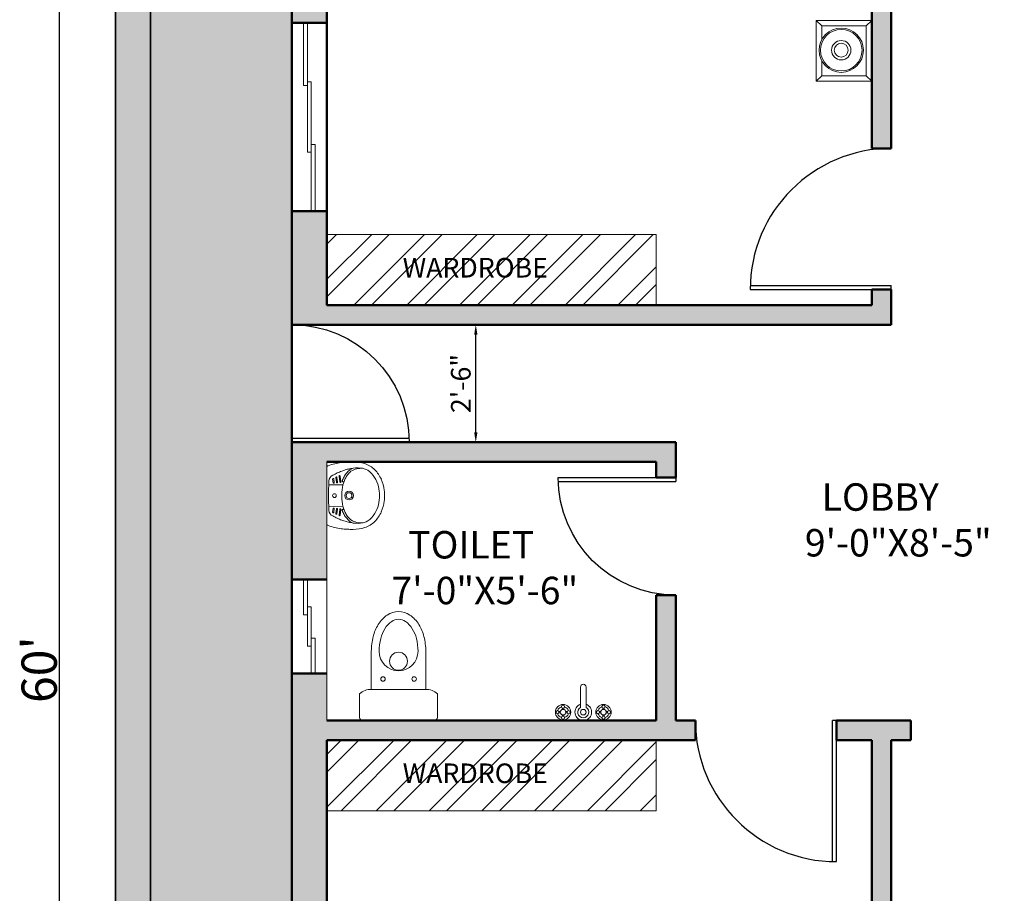
# Model space of a CAD drawing. Units: inches. Extents: x 1734 to 4011, y 1071 to 1891.
# Tile 3 of 27: x 1734 to 1985, y 1427 to 1650. Entities that reach past the tile are written whole.
import ezdxf

# ---------------------------------------------------------------- set-up
doc = ezdxf.new("R2010")
doc.units = ezdxf.units.IN
for name, color, linetype, lineweight in [('0.15', 34, 'Continuous', 15), ('A-ANNO-DIMS', 2, 'Continuous', 18), ('A-AREA-IDEN', 3, 'Continuous', 18), ('A-DOOR', 3, 'Continuous', 25), ('A-FLOR-FIXT', 9, 'Continuous', 18), ('A-FLOR-PATT', 252, 'Continuous', 13), ('A-FURN', 8, 'Continuous', 18), ('A-FURN-PATT', 252, 'Continuous', 13), ('A-GLAZ', 4, 'Continuous', 18), ('A-WALL', 7, 'Continuous', 50), ('A-WALL-PATT', 8, 'Continuous', 13), ('C-PROP', 1, 'Continuous', 35)]:
    doc.layers.add(name, color=color, linetype=linetype, lineweight=lineweight)
doc.styles.get("Standard").update_dxf_attribs({"font": 'arial.ttf'})
doc.dimstyles.new('ISO-25', dxfattribs={"dimtxt": 5, "dimasz": 2.5, "dimexe": 1.25, "dimexo": 0.625, "dimtad": 1, "dimdec": 1, "dimlunit": 3, "dimtxsty": 'Standard', "dimcen": 2.5, "dimclrt": 1, "dimadec": 0, "dimazin": 0, "dimtfac": 1, "dimtdec": 1, "dimtmove": 0, "dimatfit": 3, "dimfxl": 1, "dimarcsym": 0})

# ---------------------------------------------------------------- blocks, each defined once
blk = doc.blocks.new('*D1')
at = {"layer": 'A-ANNO-DIMS', "color": 0, "lineweight": -2, "transparency": 16777216}
for p, q in [((1850.54, 1572.06), (1849.37, 1572.06)), ((1850.62, 1544.56), (1850.62, 1569.56)), ((1850.54, 1542.06), (1849.37, 1542.06))]:
    blk.add_line(p, q, dxfattribs=at)
at = {"layer": 'A-ANNO-DIMS', "color": 0, "transparency": 16777216}
for points in [[(1850.21, 1569.56), (1851.04, 1569.56), (1850.62, 1572.06)], [(1850.21, 1544.56), (1851.04, 1544.56), (1850.62, 1542.06)]]:
    blk.add_solid(points, dxfattribs=at)
at = {"layer": 'Defpoints', "color": 0, "transparency": 16777216}
for p in [(1850.62, 1572.06), (1851.16, 1572.06), (1851.16, 1542.06)]:
    blk.add_point(p, dxfattribs=at)
at = {"layer": 'A-ANNO-DIMS', "color": 0, "transparency": 16777216, "insert": (1847.45, 1557.06), "char_height": 5, "attachment_point": 5, "rotation": 90}
blk.add_mtext('2\'-6"', dxfattribs=at)
blk = doc.blocks.new('*D15')
at = {"layer": 'A-ANNO-DIMS', "color": 0, "lineweight": -2, "transparency": 16777216}
for p, q in [((1758.02, 1844.06), (1743.18, 1844.06)), ((1744.43, 1126.56), (1744.43, 1841.56)), ((1758.02, 1124.06), (1743.18, 1124.06))]:
    blk.add_line(p, q, dxfattribs=at)
at = {"layer": 'A-ANNO-DIMS', "color": 0, "transparency": 16777216}
for points in [[(1744.01, 1841.56), (1744.84, 1841.56), (1744.43, 1844.06)], [(1744.01, 1126.56), (1744.84, 1126.56), (1744.43, 1124.06)]]:
    blk.add_solid(points, dxfattribs=at)
at = {"layer": 'Defpoints', "color": 0, "transparency": 16777216}
for p in [(1744.43, 1844.06), (1758.65, 1844.06), (1758.65, 1124.06)]:
    blk.add_point(p, dxfattribs=at)
at = {"layer": 'A-ANNO-DIMS', "color": 0, "transparency": 16777216, "insert": (1739.21, 1484.06), "char_height": 5, "attachment_point": 5, "rotation": 90}
blk.add_mtext("{\\H1.8x;60'}", dxfattribs=at)
blk = doc.blocks.new("D1 3'")
for p, q in [((0, 36), (0, 0)), ((1, 36), (1, 0)), ((0, 0), (1, 0))]:
    blk.add_line(p, q)
blk.add_arc((0, 0), 36, 0, 90)
blk = doc.blocks.new("D2 2'6")
for p, q in [((0, 30), (0, 0)), ((1, 30), (1, 0)), ((0, 0), (1, 0))]:
    blk.add_line(p, q)
blk.add_arc((0, 0), 30, 0, 90)
blk = doc.blocks.new('VELADOR')
at = {"layer": '0.15'}
for p, q in [((-0.2475, 0), (-0.2025, -0.045)), ((0.2475, 0), (0.2025, -0.045)), ((-0.2025, -0.405), (-0.2475, -0.45)), ((0.2475, -0.45), (0.2025, -0.405))]:
    blk.add_line(p, q, dxfattribs=at)
blk.add_lwpolyline([(-0.2475, 0), (-0.2475, -0.45), (0.2475, -0.45), (0.2475, 0)], close=True, dxfattribs=at)
blk.add_lwpolyline([(0.0921, -0.405), (0.2025, -0.405), (0.2025, -0.045), (-0.2025, -0.045), (-0.2025, -0.405), (-0.0818, -0.405)], dxfattribs=at)
for radius in [0.18, 0.1688, 0.0788, 0.0563]:
    blk.add_circle((0.0052, -0.2474), radius, dxfattribs=at)
blk = doc.blocks.new('lavamanos 2')
at = {"layer": '0.15'}
for p, q in [((0, 0.2335), (0, -0.2335)), ((-0.1304, 0.11), (-0.1315, 0.11)), ((-0.0142, 0.087), (-0.13, 0.086)), ((-0.1127, 0.112), (-0.1067, 0.1581)), ((-0.1037, 0.1109), (-0.0978, 0.157)), ((-0.0857, 0.1085), (-0.0807, 0.1466)), ((-0.0767, 0.1074), (-0.0718, 0.1455)), ((-0.0587, 0.105), (-0.0548, 0.1351)), ((-0.0497, 0.1039), (-0.0458, 0.134)), ((-0.1304, -0.11), (-0.1315, -0.11)), ((-0.0142, -0.087), (-0.13, -0.086)), ((-0.1127, -0.112), (-0.1067, -0.1581)), ((-0.1037, -0.1109), (-0.0978, -0.157)), ((-0.0857, -0.1085), (-0.0807, -0.1466)), ((-0.0767, -0.1074), (-0.0718, -0.1455)), ((-0.0587, -0.105), (-0.0548, -0.1351)), ((-0.0497, -0.1039), (-0.0458, -0.134))]:
    blk.add_line(p, q, dxfattribs=at)
for centre, radius in [((-0.178, 0), 0.035), ((-0.178, 0), 0.0235), ((-0.06, 0), 0.015)]:
    blk.add_circle(centre, radius, dxfattribs=at)
for centre, radius, start, end in [((-0.2419, 0.0663), 0.2023, 108.1945, 135.36859), ((-0.2035, -0.0862), 0.3593, 91.20299, 106.42552), ((-0.2208, -0.6855), 0.9585, 86.55138, 89.41308), ((-0.2121, -0.5476), 0.8204, 83.12241, 86.5796), ((5.8279, 30.215), 30.5319, 258.77821, 258.87599), ((-0.1265, -0.0657), 0.3287, 69.06009, 78.82181), ((-0.0202, 0.212), 0.0314, 54.79491, 69.06009), ((-0.1663, 0.0005), 0.3024, 136.57187, 154.32772), ((-0.2422, 0.0655), 0.1638, 121.99295, 150.58892), ((-0.2657, 0.1037), 0.119, 92.47742, 122.14108), ((-0.2765, 0.0677), 0.1528, 57.2491, 95.54005), ((-0.2442, -0.0128), 0.2368, 77.24819, 96.46321), ((-0.2765, 0.0677), 0.1678, 56.87663, 64.99714), ((-0.3662, -0.002), 0.2627, 40.35252, 49.00458), ((-0.2222, 0.0026), 0.2177, 71.98488, 82.01242), ((-0.3662, -0.002), 0.2777, 40.35252, 49.22548), ((-0.2374, 0.11), 0.0921, 27.31862, 39.11562), ((-0.3103, -0.315), 0.5472, 69.51913, 73.49118), ((-0.2374, 0.11), 0.1071, 27.57433, 39.11562), ((-0.3494, 0.0363), 0.2408, 22.19214, 30.78376), ((-0.2991, -0.2855), 0.5156, 65.23004, 69.53785), ((-0.1022, 0.1575), 0.0045, 352.61396, 172.61396), ((-0.2784, -0.2408), 0.4663, 60.24131, 65.2382), ((-0.0648, 0.1184), 0.049, 1.58272, 68.62081), ((-0.005, 0.2335), 0.005, 0, 54.79491), ((-0.0557, -0.0178), 0.4111, 158.70106, 171.31016), ((-0.1999, 0.0263), 0.2202, 147.11565, 167.44248), ((-0.3494, 0.0363), 0.2258, 22.33605, 30.8927), ((-1.2664, -0.2389), 1.1824, 16.36313, 17.77674), ((-0.1315, 0.117), 0.007, 197.40991, 270.49494), ((0.1853, 0.1648), 0.325, 192.53887, 196.70718), ((-0.1305, 0.117), 0.007, 270.49494, 17.39527), ((-1.2664, -0.2389), 1.1974, 17.39527, 17.80495), ((-0.1082, 0.1115), 0.0045, 172.61396, 352.61396), ((-0.0812, 0.108), 0.0045, 172.61396, 352.61396), ((-0.0763, 0.146), 0.0045, 352.61396, 172.61396), ((-0.0542, 0.1045), 0.0045, 172.61396, 352.61396), ((-0.0503, 0.1345), 0.0045, 352.61396, 172.61396), ((-2.1477, 0.0009), 2.1352, 359.97535, 3.19009), ((-0.2093, 0.0056), 0.2558, 171.31016, 181.26266), ((-0.2093, -0.0056), 0.2558, 178.73734, 188.68984), ((0.4664, -0.0834), 0.8953, 169.86317, 174.65802), ((0.4664, 0.0834), 0.8953, 185.34198, 190.13683), ((0.3887, 0.121), 0.517, 185.50529, 189.81306), ((-0.7181, -0.0071), 0.5987, 0.67647, 3.82165), ((-0.7181, 0.0071), 0.5987, 356.17835, 359.32353), ((-2.1477, -0.0009), 2.1352, 356.80991, 0.02465), ((-0.0557, 0.0178), 0.4111, 188.68984, 201.29894), ((-0.1999, -0.0263), 0.2202, 192.55752, 212.88435), ((0.1853, -0.1648), 0.325, 163.29282, 167.46113), ((0.3887, -0.1209), 0.517, 170.18694, 174.49471), ((-0.1663, -0.0005), 0.3024, 205.67228, 223.42813), ((-0.2422, -0.0655), 0.1638, 209.41108, 238.00705), ((-0.2374, -0.1099), 0.0921, 320.88438, 332.68138), ((-0.3494, -0.0363), 0.2258, 329.1073, 337.66395), ((-0.3494, -0.0363), 0.2408, 329.21624, 337.80786), ((-1.2664, 0.2389), 1.1824, 342.22326, 343.63687), ((-0.1315, -0.117), 0.007, 89.50506, 162.59009), ((-0.1305, -0.117), 0.007, 342.60473, 89.50506), ((-1.2664, 0.2389), 1.1974, 342.19505, 342.60473), ((-0.1082, -0.1115), 0.0045, 7.38604, 187.38604), ((-0.1022, -0.1575), 0.0045, 187.38604, 7.38604), ((-0.0812, -0.108), 0.0045, 7.38604, 187.38604), ((-0.0763, -0.146), 0.0045, 187.38604, 7.38604), ((-0.0542, -0.1045), 0.0045, 7.38604, 187.38604), ((-0.0503, -0.1345), 0.0045, 187.38604, 7.38604), ((-0.0648, -0.1184), 0.049, 291.37919, 358.41728), ((-0.2419, -0.0663), 0.2023, 224.63141, 251.8055), ((-0.2657, -0.1036), 0.119, 237.85892, 267.52258), ((-0.2765, -0.0677), 0.1528, 264.45995, 302.7509), ((-0.2442, 0.0128), 0.2368, 263.53679, 282.75181), ((-0.2765, -0.0677), 0.1678, 295.00286, 303.12337), ((-0.3662, 0.002), 0.2627, 310.99542, 319.64748), ((-0.2222, -0.0026), 0.2177, 277.98758, 288.01512), ((-0.3662, 0.002), 0.2777, 310.77452, 319.64748), ((-0.3103, 0.315), 0.5472, 286.50882, 290.48087), ((-0.2374, -0.1099), 0.1071, 320.88438, 332.42567), ((-0.2991, 0.2855), 0.5156, 290.46215, 294.76996), ((-0.2784, 0.2408), 0.4663, 294.7618, 299.75869), ((-0.0202, -0.212), 0.0314, 290.93991, 305.20509), ((-0.005, -0.2335), 0.005, 305.20509, 0), ((-0.2035, 0.0862), 0.3593, 253.57448, 268.79701), ((-0.2208, 0.6855), 0.9585, 270.58692, 273.44862), ((-0.2121, 0.5476), 0.8204, 273.4204, 276.87759), ((5.8279, -30.215), 30.5319, 101.12401, 101.22179), ((-0.1265, 0.0657), 0.3287, 281.17819, 290.93991)]:
    blk.add_arc(centre, radius, start, end, dxfattribs=at)
blk = doc.blocks.new('rreerr')
blk.add_lwpolyline([(2512.8529, 833.5601, 0.205217), (2512.9279, 833.5883), (2512.9279, 833.7401, 0.414214), (2512.9079, 833.7601), (2512.4479, 833.7601, 0.414214), (2512.4279, 833.7401), (2512.4279, 833.5883, 0.205217), (2512.5029, 833.5601)], format="xyb")
for points in [[(2512.5468, 833.1438, 0.107027), (2512.6056, 833.0819, 0.150548), (2512.6779, 833.0596, 0.150548), (2512.7502, 833.0819, 0.107027), (2512.809, 833.1438, 0.075071), (2512.8412, 833.2206, 0.0618), (2512.8529, 833.3151), (2512.8529, 833.5601), (2512.5029, 833.5601), (2512.5029, 833.3151, 0.0618), (2512.5146, 833.2206, 0.075071)], [(2512.5631, 833.2328, 0.075071), (2512.5895, 833.1698, 0.107027), (2512.6338, 833.1232, 0.150548), (2512.6779, 833.1096, 0.150548), (2512.722, 833.1232, 0.107027), (2512.7663, 833.1698, 0.075071), (2512.7927, 833.2328, 0.0618), (2512.8029, 833.3151, 1), (2512.5529, 833.3151, 0.0618)]]:
    blk.add_lwpolyline(points, format="xyb", close=True)
for centre, radius in [((2512.5779, 833.493), 0.0146), ((2512.7779, 833.493), 0.0146), ((2512.6775, 833.3793), 0.0579)]:
    blk.add_circle(centre, radius)
blk = doc.blocks.new('Faucet - Bathroom top')
for p, q in [((-4.107, 0.125), (-4.375, 0.125)), ((-3.75, 0.4788), (-3.75, 0.75)), ((-3.5, 0.482), (-3.5, 0.75)), ((-3.1461, 0.125), (-2.875, 0.125)), ((3.143, 0.125), (2.875, 0.125)), ((3.5, 0.4788), (3.5, 0.75)), ((3.75, 0.482), (3.75, 0.75)), ((4.1039, 0.125), (4.375, 0.125)), ((-4.1039, -0.125), (-4.375, -0.125)), ((-3.75, -0.4821), (-3.75, -0.75)), ((-3.5, -0.4789), (-3.5, -0.75)), ((-3.143, -0.125), (-2.875, -0.125)), ((-0.5, -0.8639), (-0.5, -4.5)), ((0.5, -4.5), (0.5, -0.8631)), ((3.1461, -0.125), (2.875, -0.125)), ((3.5, -0.4821), (3.5, -0.75)), ((3.75, -0.4789), (3.75, -0.75)), ((4.107, -0.125), (4.375, -0.125))]:
    blk.add_line(p, q)
for centre, radius in [((-3.625, 0), 1.375), ((-4.625, 0), 0.2795), ((-3.625, 0), 0.5), ((-3.625, 1), 0.2795), ((-2.625, 0), 0.2795), ((0, 0), 0.5), ((3.625, 0), 1.375), ((2.625, 0), 0.2795), ((3.625, 0), 0.5), ((3.625, 1), 0.2795), ((4.625, 0), 0.2795), ((-3.625, -1), 0.2795), ((3.625, -1), 0.2795)]:
    blk.add_circle(centre, radius)
for centre, radius, start, end in [((-3.625, 0), 1, 105.2407, 164.2093), ((-3.625, 0), 1, 16.44125, 74.07887), ((0, 0), 1.5, 289.6514, 250.3603), ((0, 0), 1, 300.3431, 239.7554), ((3.625, 0), 1, 106.12, 164.0884), ((3.625, 0), 1, 16.23422, 73.90469), ((-3.625, 0), 1, 196.2342, 253.9047), ((-3.625, 0), 1, 286.12, 344.0884), ((3.625, 0), 1, 196.4413, 254.0789), ((3.625, 0), 1, 285.2407, 344.2093), ((0, -4.5), 0.5, 180, 0)]:
    blk.add_arc(centre, radius, start, end)

msp = doc.modelspace()

# ---------------------------------------------------------------- hatches: boundary and pattern name
at = {"layer": 'A-FLOR-PATT'}
h = msp.add_hatch(color=256, dxfattribs=at)
h.dxf.hatch_style = 1
h.paths.add_polyline_path([(1767.65, 1758.06), (1758.65, 1758.06), (1758.65, 1124.06), (1814.65, 1124.06), (1814.65, 1133.06), (1767.65, 1133.06)])
h = msp.add_hatch(color=256, dxfattribs=at)
h.dxf.hatch_style = 1
h.paths.add_polyline_path([(1803.65, 1758.06), (1767.65, 1758.06), (1767.65, 1325.06), (1803.65, 1325.06), (1803.65, 1542.06)])
at = {"layer": 'A-FURN-PATT'}
h = msp.add_hatch(dxfattribs=at)
h.set_pattern_fill('ANSI32', color=256)
h.paths.add_polyline_path([(1951.65, 1835.06), (1862.65, 1835.06), (1862.65, 1817.06), (1951.65, 1817.06)])
h.paths.add_polyline_path([(1896.65, 1466.06), (1812.65, 1466.06), (1812.65, 1448.06), (1896.65, 1448.06)])
h.paths.add_polyline_path([(1826.14, 1452.28), (1875.6, 1452.28), (1875.6, 1462.58), (1826.14, 1462.58)], flags=24)
h = msp.add_hatch(dxfattribs=at)
h.set_pattern_fill('ANSI32', color=256)
h.paths.add_polyline_path([(1896.65, 1595.06), (1812.65, 1595.06), (1812.65, 1577.06), (1896.65, 1577.06)])
h.paths.add_polyline_path([(1826.14, 1581.28), (1875.6, 1581.28), (1875.6, 1591.58), (1826.14, 1591.58)], flags=24)
at = {"layer": 'A-WALL-PATT'}
h = msp.add_hatch(color=256, dxfattribs=at)
h.dxf.hatch_style = 1
h.paths.add_polyline_path([(1857.65, 1835.06), (1857.65, 1793.06), (1862.65, 1793.06), (1862.65, 1835.06), (1951.65, 1835.06), (1951.65, 1763.06), (1897.65, 1763.06), (1897.65, 1758.06), (1951.65, 1758.06), (1951.65, 1617.06), (1956.65, 1617.06), (1956.65, 1758.06), (2009.65, 1758.06), (2009.65, 1763.06), (1956.65, 1763.06), (1956.65, 1835.06), (2044.65, 1835.06), (2044.65, 1763.06), (2039.65, 1763.06), (2039.65, 1758.06), (2054.65, 1758.06), (2054.65, 1763.06), (2049.65, 1763.06), (2049.65, 1835.06), (2109.65, 1835.06), (2109.65, 1763.06), (2084.65, 1763.06), (2084.65, 1758.06), (2109.65, 1758.06), (2109.65, 1530.06), (2095.15, 1530.06), (2095.15, 1525.06), (2109.65, 1525.06), (2109.65, 1471.06), (2089.15, 1471.06), (2089.15, 1466.06), (2109.65, 1466.06), (2109.65, 1250.06), (2015.65, 1250.06), (2015.65, 1241.06), (2109.65, 1241.06), (2109.65, 1133.06), (1952.65, 1133.06), (1952.65, 1197.06), (1953.65, 1197.06), (1953.65, 1202.06), (1946.65, 1202.06), (1946.65, 1133.06), (1934.65, 1133.06), (1934.65, 1124.06), (2118.65, 1124.06), (2118.65, 1844.06), (1758.65, 1844.06), (1758.65, 1758.06), (1773.65, 1758.06), (1773.65, 1763.06), (1767.65, 1763.06), (1767.65, 1835.06)])
h.paths.add_polyline_path([(1803.65, 1649.06), (1812.65, 1649.06), (1812.65, 1758.06), (1867.65, 1758.06), (1867.65, 1763.06), (1797.65, 1763.06), (1797.65, 1758.06), (1803.65, 1758.06)], flags=17)
h.paths.add_polyline_path([(1803.65, 1572.06), (1956.65, 1572.06), (1956.65, 1581.06), (1951.65, 1581.06), (1951.65, 1577.06), (1812.65, 1577.06), (1812.65, 1601.06), (1803.65, 1601.06)], flags=17)
h.paths.add_polyline_path([(2044.65, 1530.06), (2044.65, 1525.06), (2059.15, 1525.06), (2059.15, 1530.06)], flags=17)
h.paths.add_polyline_path([(2009.65, 1466.06), (2035.15, 1466.06), (2035.15, 1471.06), (2014.65, 1471.06), (2014.65, 1530.06), (2009.65, 1530.06)], flags=17)
h.paths.add_polyline_path([(1896.65, 1537.06), (1896.65, 1533.06), (1901.65, 1533.06), (1901.65, 1542.06), (1803.65, 1542.06), (1803.65, 1507.06), (1812.65, 1507.06), (1812.65, 1537.06)], flags=17)
h.paths.add_polyline_path([(1906.65, 1466.06), (1906.65, 1471.06), (1901.65, 1471.06), (1901.65, 1503.06), (1896.65, 1503.06), (1896.65, 1471.06), (1812.65, 1471.06), (1812.65, 1483.06), (1803.65, 1483.06), (1803.65, 1400.06), (1812.65, 1400.06), (1812.65, 1466.06)], flags=17)
h.paths.add_polyline_path([(1951.65, 1334.06), (1909.15, 1334.06), (1909.15, 1325.06), (1956.65, 1325.06), (1956.65, 1466.06), (1961.65, 1466.06), (1961.65, 1471.06), (1942.65, 1471.06), (1942.65, 1466.06), (1951.65, 1466.06)], flags=17)
h.paths.add_polyline_path([(1812.65, 1334.06), (1812.65, 1352.06), (1803.65, 1352.06), (1803.65, 1325.06), (1855.15, 1325.06), (1855.15, 1334.06)], flags=17)
h.paths.add_polyline_path([(1956.65, 1298.06), (1956.65, 1301.06), (1947.65, 1301.06), (1947.65, 1298.06)], flags=17)
h.paths.add_polyline_path([(1967.65, 1241.06), (1967.65, 1250.06), (1947.65, 1250.06), (1947.65, 1241.06)], flags=17)

# ---------------------------------------------------------------- linework, layer by layer
at = {"layer": 'A-FURN'}
for p, q in [((1812.65, 1595.06), (1896.65, 1595.06)), ((1896.65, 1577.06), (1896.65, 1595.06)), ((1812.65, 1471.06), (1812.65, 1537.06)), ((1812.65, 1448.06), (1896.65, 1448.06))]:
    msp.add_line(p, q, dxfattribs=at)
at = {"layer": 'A-GLAZ'}
for p, q in [((1806.65, 1649.06), (1806.65, 1633.06)), ((1807.65, 1649.06), (1807.65, 1616.06)), ((1807.65, 1634.06), (1808.65, 1634.06)), ((1808.65, 1634.06), (1808.65, 1601.06)), ((1806.65, 1633.06), (1807.65, 1633.06)), ((1808.65, 1618.06), (1809.65, 1618.06)), ((1809.65, 1618.06), (1809.65, 1601.06)), ((1807.65, 1616.06), (1808.65, 1616.06)), ((1806.65, 1498.06), (1806.65, 1507.06)), ((1807.65, 1490.06), (1807.65, 1507.06)), ((1808.65, 1500.06), (1807.65, 1500.06)), ((1808.65, 1483.06), (1808.65, 1500.06)), ((1807.65, 1498.06), (1806.65, 1498.06)), ((1808.65, 1490.06), (1807.65, 1490.06)), ((1809.65, 1492.06), (1808.65, 1492.06)), ((1809.65, 1483.06), (1809.65, 1492.06)), ((1896.65, 1448.06), (1896.65, 1466.06))]:
    msp.add_line(p, q, dxfattribs=at)
at = {"layer": 'A-WALL'}
for p, q in [((1803.65, 1542.06), (1803.65, 1758.06)), ((1812.65, 1577.06), (1812.65, 1758.06)), ((1951.65, 1617.06), (1951.65, 1758.06)), ((1956.65, 1617.06), (1956.65, 1758.06)), ((1803.65, 1649.06), (1812.65, 1649.06)), ((1951.65, 1617.06), (1956.65, 1617.06)), ((1803.65, 1601.06), (1812.65, 1601.06)), ((1951.65, 1577.06), (1951.65, 1581.06)), ((1951.65, 1581.06), (1956.65, 1581.06)), ((1956.65, 1572.06), (1956.65, 1581.06)), ((1812.65, 1577.06), (1951.65, 1577.06)), ((1812.65, 1577.06), (1896.65, 1577.06)), ((1803.65, 1572.06), (1956.65, 1572.06)), ((1803.65, 1325.06), (1803.65, 1542.06)), ((1803.65, 1542.06), (1901.65, 1542.06)), ((1901.65, 1533.06), (1901.65, 1542.06)), ((1812.65, 1537.06), (1896.65, 1537.06)), ((1896.65, 1533.06), (1896.65, 1537.06)), ((1896.65, 1533.06), (1901.65, 1533.06)), ((1812.65, 1507.06), (1803.65, 1507.06)), ((1896.65, 1503.06), (1901.65, 1503.06)), ((1896.65, 1471.06), (1896.65, 1503.06)), ((1901.65, 1471.06), (1901.65, 1503.06)), ((1812.65, 1483.06), (1803.65, 1483.06)), ((1812.65, 1471.06), (1896.65, 1471.06)), ((1901.65, 1471.06), (1906.65, 1471.06)), ((1906.65, 1466.06), (1906.65, 1471.06)), ((1942.65, 1466.06), (1942.65, 1471.06)), ((1942.65, 1471.06), (1961.65, 1471.06)), ((1961.65, 1466.06), (1961.65, 1471.06)), ((1812.65, 1466.06), (1906.65, 1466.06)), ((1812.65, 1334.06), (1812.65, 1466.06)), ((1942.65, 1466.06), (1951.65, 1466.06)), ((1951.65, 1334.06), (1951.65, 1466.06)), ((1956.65, 1298.06), (1956.65, 1466.06)), ((1956.65, 1466.06), (1961.65, 1466.06))]:
    msp.add_line(p, q, dxfattribs=at)
at = {"layer": 'C-PROP'}
msp.add_line((1767.65, 1133.06), (1767.65, 1758.06), dxfattribs=at)
msp.add_lwpolyline([(1814.65, 1124.06), (1758.65, 1124.06), (1758.65, 1844.06), (2118.65, 1844.06), (2118.65, 1124.06), (1934.65, 1124.06)], dxfattribs=at)

# ---------------------------------------------------------------- block references
at = {"layer": 'A-DOOR'}
for p, rotation in [((1956.65, 1581.06), 90), ((1942.65, 1471.06), 180)]:
    msp.add_blockref("D1 3'", p, dxfattribs=dict(at, rotation=rotation))
at = {"layer": 'A-DOOR', "xscale": -1}
for p, rotation in [((1803.65, 1542.06), 270), ((1901.65, 1533.06), 90)]:
    msp.add_blockref("D2 2'6", p, dxfattribs=dict(at, rotation=rotation))
at = {"layer": 'A-FLOR-FIXT'}
for name, p, xscale, yscale, zscale, rotation in [('lavamanos 2', (1812.65, 1528.45), 31.61240364394164, 31.61240364394164, 31.61240364394164, 179.99990349049), ('rreerr', (-97924.91, 34572.17), -39.701, 39.701, 39.701, 180), ('Faucet - Bathroom top', (1878.05, 1473.2), -1.424049708253414, 1.424049708253414, 1.424049708253414, 180)]:
    msp.add_blockref(name, p, dxfattribs=dict(at, xscale=xscale, yscale=yscale, zscale=zscale, rotation=rotation))
at = {"layer": 'A-FURN', "xscale": -31.41542173157097, "yscale": 31.41542173157097, "zscale": 31.41542173157097, "rotation": 269.9999999999999}
msp.add_blockref('VELADOR', (1951.65, 1641.94), dxfattribs=at)

# ---------------------------------------------------------------- texts
at = {"layer": 'A-AREA-IDEN', "attachment_point": 1}
for s, insert, char_height in [('   WARDROBE', (1827.39, 1589.1), 5), ('  LOBBY\\P9\'-0"X8\'-5"', (1934.59, 1531.59), 7), ('  TOILET\\P7\'-0"X5\'-6"', (1829.1, 1519.41), 7), ('   WARDROBE', (1827.39, 1460.1), 5)]:
    msp.add_mtext_dynamic_manual_height_columns(s, width=86.9528, gutter_width=12.5, heights=[0], dxfattribs=dict(at, insert=insert, char_height=char_height))

# ---------------------------------------------------------------- dimensions: what is measured, and where the dimension line sits
at = {"layer": 'A-ANNO-DIMS'}
dim = msp.add_linear_dim(base=(1744.43, 1844.06), p1=(1758.65, 1124.06), p2=(1758.65, 1844.06), angle=90, text='{\\H1.8x;<>}', dimstyle='ISO-25', override={"dimclrd": 0, "dimclre": 0, "dimclrt": 0}, dxfattribs=at)
dim.commit()
dim.dimension.update_dxf_attribs({"geometry": '*D15', "text_midpoint": (1739.21, 1484.06)})
dim = msp.add_linear_dim(base=(1850.62, 1572.06), p1=(1851.16, 1542.06), p2=(1851.16, 1572.06), angle=90, dimstyle='ISO-25', override={"dimclrd": 0, "dimclre": 0, "dimclrt": 0}, dxfattribs=at)
dim.commit()
dim.dimension.update_dxf_attribs({"geometry": '*D1', "text_midpoint": (1847.45, 1557.06)})

doc.saveas('drawing.dxf')
